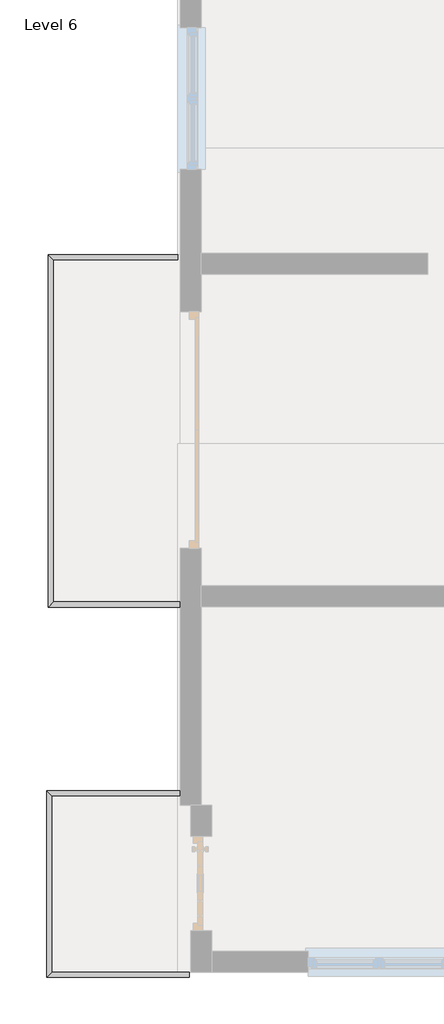
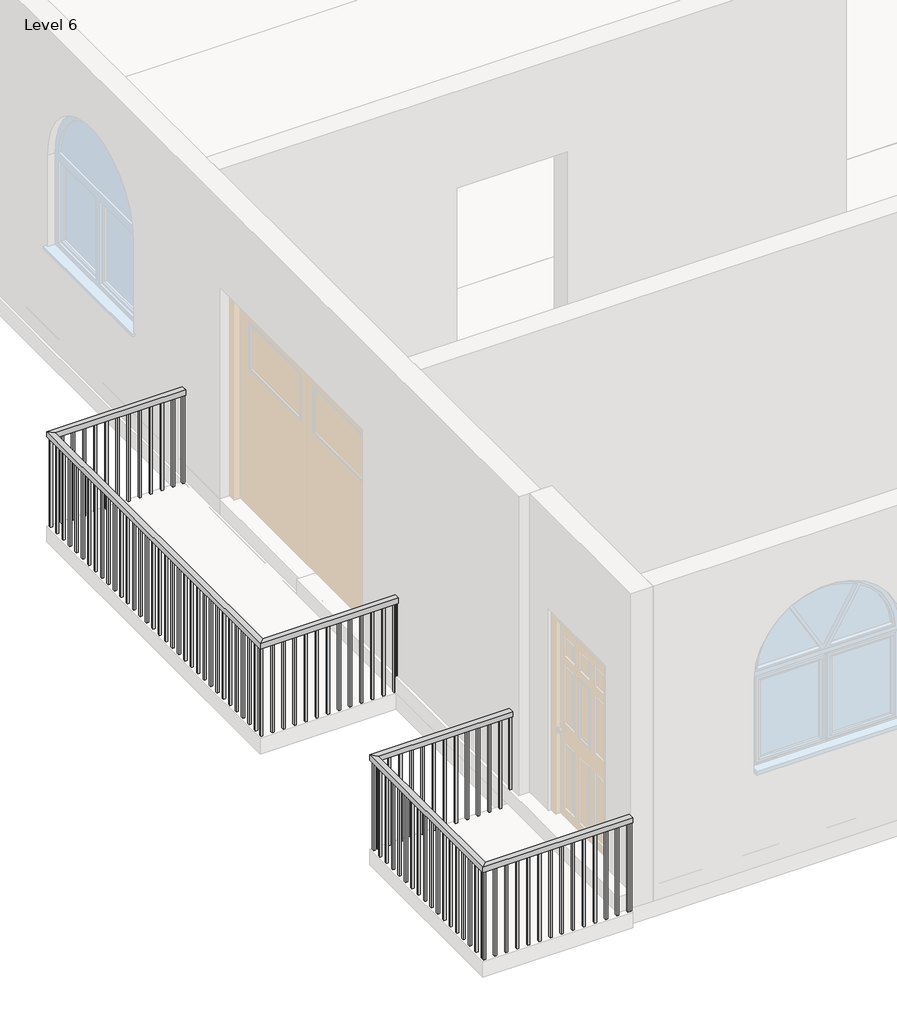
# One storey, part 3 of 7: 2 railings.
"""IFC4 building model written with IfcOpenShell, lengths in millimetres."""

from ifc_helpers import new_model, si_unit, frame, origin, place, context, project, spatial, polyline, outline, extrude, faceted_brep, element, save

model = new_model("IFC4")

# Units and contexts
model_context = context("Model", 3, world=origin())
ifc_project = project(units=[si_unit("LENGTHUNIT", "METRE", prefix="MILLI")], contexts=[model_context])

# Site, building, storey
site = spatial("IfcSite", under=ifc_project)
building = spatial("IfcBuilding", under=site)
storey = spatial("IfcBuildingStorey", under=building, Name="Level 6", Elevation=15240.0)

# Railings
placement = place(None, origin())
element("IfcRailing", 1, ObjectType="Handrail - Rectangular", at=placement, inside=storey, context=model_context, shape_type="SolidModel", body=[
    faceted_brep([(-6354.2109037, -3767.6037749, 16154.4), (-6354.2109037, -3767.6037749, 16103.6), (-6354.2109037, -3716.8037749, 16103.6), (-6354.2109037, -3716.8037749, 16154.4), (-7548.0109037, -3767.6037749, 16154.4), (-7548.0109037, -3767.6037749, 16103.6), (-7598.8109037, -3716.8037749, 16103.6), (-7598.8109037, -3716.8037749, 16154.4), (-7548.0109037, -7054.4894702, 16154.4), (-7548.0109037, -7054.4894702, 16103.6), (-7598.8109037, -7105.2894702, 16103.6), (-7598.8109037, -7105.2894702, 16154.4), (-6330.8013636, -7054.4894702, 16154.4), (-6330.8013636, -7105.2894702, 16154.4), (-6330.8013636, -7105.2894702, 16103.6), (-6330.8013636, -7054.4894702, 16103.6)], [[[0, 1, 2, 3]], [[1, 0, 4, 5]], [[2, 1, 5, 6]], [[3, 2, 6, 7]], [[0, 3, 7, 4]], [[5, 4, 8, 9]], [[6, 5, 9, 10]], [[7, 6, 10, 11]], [[4, 7, 11, 8]], [[12, 13, 14, 15]], [[9, 8, 12, 15]], [[10, 9, 15, 14]], [[11, 10, 14, 13]], [[8, 11, 13, 12]]]),
    extrude(outline(polyline([(-6363.7359037, -7089.4144702), (-6363.7359037, -7070.3644702), (-6344.6859037, -7070.3644702), (-6344.6859037, -7089.4144702), (-6363.7359037, -7089.4144702)])), frame((0.0, 0.0, 15240.0), z_axis=(0.0, 0.0, 1.0), x_axis=(1.0, 0.0, 0.0)), (0.0, 0.0, 1.0), 863.6),
    extrude(outline(polyline([(-6465.3359037, -7089.4144702), (-6465.3359037, -7070.3644702), (-6446.2859037, -7070.3644702), (-6446.2859037, -7089.4144702), (-6465.3359037, -7089.4144702)])), frame((0.0, 0.0, 15240.0), z_axis=(0.0, 0.0, 1.0), x_axis=(1.0, 0.0, 0.0)), (0.0, 0.0, 1.0), 863.6),
    extrude(outline(polyline([(-6566.9359037, -7089.4144702), (-6566.9359037, -7070.3644702), (-6547.8859037, -7070.3644702), (-6547.8859037, -7089.4144702), (-6566.9359037, -7089.4144702)])), frame((0.0, 0.0, 15240.0), z_axis=(0.0, 0.0, 1.0), x_axis=(1.0, 0.0, 0.0)), (0.0, 0.0, 1.0), 863.6),
    extrude(outline(polyline([(-6668.5359037, -7089.4144702), (-6668.5359037, -7070.3644702), (-6649.4859037, -7070.3644702), (-6649.4859037, -7089.4144702), (-6668.5359037, -7089.4144702)])), frame((0.0, 0.0, 15240.0), z_axis=(0.0, 0.0, 1.0), x_axis=(1.0, 0.0, 0.0)), (0.0, 0.0, 1.0), 863.6),
    extrude(outline(polyline([(-6770.1359037, -7089.4144702), (-6770.1359037, -7070.3644702), (-6751.0859037, -7070.3644702), (-6751.0859037, -7089.4144702), (-6770.1359037, -7089.4144702)])), frame((0.0, 0.0, 15240.0), z_axis=(0.0, 0.0, 1.0), x_axis=(1.0, 0.0, 0.0)), (0.0, 0.0, 1.0), 863.6),
    extrude(outline(polyline([(-6871.7359037, -7089.4144702), (-6871.7359037, -7070.3644702), (-6852.6859037, -7070.3644702), (-6852.6859037, -7089.4144702), (-6871.7359037, -7089.4144702)])), frame((0.0, 0.0, 15240.0), z_axis=(0.0, 0.0, 1.0), x_axis=(1.0, 0.0, 0.0)), (0.0, 0.0, 1.0), 863.6),
    extrude(outline(polyline([(-6973.3359037, -7089.4144702), (-6973.3359037, -7070.3644702), (-6954.2859037, -7070.3644702), (-6954.2859037, -7089.4144702), (-6973.3359037, -7089.4144702)])), frame((0.0, 0.0, 15240.0), z_axis=(0.0, 0.0, 1.0), x_axis=(1.0, 0.0, 0.0)), (0.0, 0.0, 1.0), 863.6),
    extrude(outline(polyline([(-7074.9359037, -7089.4144702), (-7074.9359037, -7070.3644702), (-7055.8859037, -7070.3644702), (-7055.8859037, -7089.4144702), (-7074.9359037, -7089.4144702)])), frame((0.0, 0.0, 15240.0), z_axis=(0.0, 0.0, 1.0), x_axis=(1.0, 0.0, 0.0)), (0.0, 0.0, 1.0), 863.6),
    extrude(outline(polyline([(-7176.5359037, -7089.4144702), (-7176.5359037, -7070.3644702), (-7157.4859037, -7070.3644702), (-7157.4859037, -7089.4144702), (-7176.5359037, -7089.4144702)])), frame((0.0, 0.0, 15240.0), z_axis=(0.0, 0.0, 1.0), x_axis=(1.0, 0.0, 0.0)), (0.0, 0.0, 1.0), 863.6),
    extrude(outline(polyline([(-7278.1359037, -7089.4144702), (-7278.1359037, -7070.3644702), (-7259.0859037, -7070.3644702), (-7259.0859037, -7089.4144702), (-7278.1359037, -7089.4144702)])), frame((0.0, 0.0, 15240.0), z_axis=(0.0, 0.0, 1.0), x_axis=(1.0, 0.0, 0.0)), (0.0, 0.0, 1.0), 863.6),
    extrude(outline(polyline([(-7379.7359037, -7089.4144702), (-7379.7359037, -7070.3644702), (-7360.6859037, -7070.3644702), (-7360.6859037, -7089.4144702), (-7379.7359037, -7089.4144702)])), frame((0.0, 0.0, 15240.0), z_axis=(0.0, 0.0, 1.0), x_axis=(1.0, 0.0, 0.0)), (0.0, 0.0, 1.0), 863.6),
    extrude(outline(polyline([(-7481.3359037, -7089.4144702), (-7481.3359037, -7070.3644702), (-7462.2859037, -7070.3644702), (-7462.2859037, -7089.4144702), (-7481.3359037, -7089.4144702)])), frame((0.0, 0.0, 15240.0), z_axis=(0.0, 0.0, 1.0), x_axis=(1.0, 0.0, 0.0)), (0.0, 0.0, 1.0), 863.6),
    extrude(outline(polyline([(-7582.9359037, -6983.8787749), (-7563.8859037, -6983.8787749), (-7563.8859037, -7002.9287749), (-7582.9359037, -7002.9287749), (-7582.9359037, -6983.8787749)])), frame((0.0, 0.0, 15240.0), z_axis=(0.0, 0.0, 1.0), x_axis=(1.0, 0.0, 0.0)), (0.0, 0.0, 1.0), 863.6),
    extrude(outline(polyline([(-7582.9359037, -6882.2787749), (-7563.8859037, -6882.2787749), (-7563.8859037, -6901.3287749), (-7582.9359037, -6901.3287749), (-7582.9359037, -6882.2787749)])), frame((0.0, 0.0, 15240.0), z_axis=(0.0, 0.0, 1.0), x_axis=(1.0, 0.0, 0.0)), (0.0, 0.0, 1.0), 863.6),
    extrude(outline(polyline([(-7582.9359037, -6780.6787749), (-7563.8859037, -6780.6787749), (-7563.8859037, -6799.7287749), (-7582.9359037, -6799.7287749), (-7582.9359037, -6780.6787749)])), frame((0.0, 0.0, 15240.0), z_axis=(0.0, 0.0, 1.0), x_axis=(1.0, 0.0, 0.0)), (0.0, 0.0, 1.0), 863.6),
    extrude(outline(polyline([(-7582.9359037, -6679.0787749), (-7563.8859037, -6679.0787749), (-7563.8859037, -6698.1287749), (-7582.9359037, -6698.1287749), (-7582.9359037, -6679.0787749)])), frame((0.0, 0.0, 15240.0), z_axis=(0.0, 0.0, 1.0), x_axis=(1.0, 0.0, 0.0)), (0.0, 0.0, 1.0), 863.6),
    extrude(outline(polyline([(-7582.9359037, -6577.4787749), (-7563.8859037, -6577.4787749), (-7563.8859037, -6596.5287749), (-7582.9359037, -6596.5287749), (-7582.9359037, -6577.4787749)])), frame((0.0, 0.0, 15240.0), z_axis=(0.0, 0.0, 1.0), x_axis=(1.0, 0.0, 0.0)), (0.0, 0.0, 1.0), 863.6),
    extrude(outline(polyline([(-7582.9359037, -6475.8787749), (-7563.8859037, -6475.8787749), (-7563.8859037, -6494.9287749), (-7582.9359037, -6494.9287749), (-7582.9359037, -6475.8787749)])), frame((0.0, 0.0, 15240.0), z_axis=(0.0, 0.0, 1.0), x_axis=(1.0, 0.0, 0.0)), (0.0, 0.0, 1.0), 863.6),
    extrude(outline(polyline([(-7582.9359037, -6374.2787749), (-7563.8859037, -6374.2787749), (-7563.8859037, -6393.3287749), (-7582.9359037, -6393.3287749), (-7582.9359037, -6374.2787749)])), frame((0.0, 0.0, 15240.0), z_axis=(0.0, 0.0, 1.0), x_axis=(1.0, 0.0, 0.0)), (0.0, 0.0, 1.0), 863.6),
    extrude(outline(polyline([(-7582.9359037, -6272.6787749), (-7563.8859037, -6272.6787749), (-7563.8859037, -6291.7287749), (-7582.9359037, -6291.7287749), (-7582.9359037, -6272.6787749)])), frame((0.0, 0.0, 15240.0), z_axis=(0.0, 0.0, 1.0), x_axis=(1.0, 0.0, 0.0)), (0.0, 0.0, 1.0), 863.6),
    extrude(outline(polyline([(-7582.9359037, -6171.0787749), (-7563.8859037, -6171.0787749), (-7563.8859037, -6190.1287749), (-7582.9359037, -6190.1287749), (-7582.9359037, -6171.0787749)])), frame((0.0, 0.0, 15240.0), z_axis=(0.0, 0.0, 1.0), x_axis=(1.0, 0.0, 0.0)), (0.0, 0.0, 1.0), 863.6),
    extrude(outline(polyline([(-7582.9359037, -6069.4787749), (-7563.8859037, -6069.4787749), (-7563.8859037, -6088.5287749), (-7582.9359037, -6088.5287749), (-7582.9359037, -6069.4787749)])), frame((0.0, 0.0, 15240.0), z_axis=(0.0, 0.0, 1.0), x_axis=(1.0, 0.0, 0.0)), (0.0, 0.0, 1.0), 863.6),
    extrude(outline(polyline([(-7582.9359037, -5967.8787749), (-7563.8859037, -5967.8787749), (-7563.8859037, -5986.9287749), (-7582.9359037, -5986.9287749), (-7582.9359037, -5967.8787749)])), frame((0.0, 0.0, 15240.0), z_axis=(0.0, 0.0, 1.0), x_axis=(1.0, 0.0, 0.0)), (0.0, 0.0, 1.0), 863.6),
    extrude(outline(polyline([(-7582.9359037, -5866.2787749), (-7563.8859037, -5866.2787749), (-7563.8859037, -5885.3287749), (-7582.9359037, -5885.3287749), (-7582.9359037, -5866.2787749)])), frame((0.0, 0.0, 15240.0), z_axis=(0.0, 0.0, 1.0), x_axis=(1.0, 0.0, 0.0)), (0.0, 0.0, 1.0), 863.6),
    extrude(outline(polyline([(-7582.9359037, -5764.6787749), (-7563.8859037, -5764.6787749), (-7563.8859037, -5783.7287749), (-7582.9359037, -5783.7287749), (-7582.9359037, -5764.6787749)])), frame((0.0, 0.0, 15240.0), z_axis=(0.0, 0.0, 1.0), x_axis=(1.0, 0.0, 0.0)), (0.0, 0.0, 1.0), 863.6),
    extrude(outline(polyline([(-7582.9359037, -5663.0787749), (-7563.8859037, -5663.0787749), (-7563.8859037, -5682.1287749), (-7582.9359037, -5682.1287749), (-7582.9359037, -5663.0787749)])), frame((0.0, 0.0, 15240.0), z_axis=(0.0, 0.0, 1.0), x_axis=(1.0, 0.0, 0.0)), (0.0, 0.0, 1.0), 863.6),
    extrude(outline(polyline([(-7582.9359037, -5561.4787749), (-7563.8859037, -5561.4787749), (-7563.8859037, -5580.5287749), (-7582.9359037, -5580.5287749), (-7582.9359037, -5561.4787749)])), frame((0.0, 0.0, 15240.0), z_axis=(0.0, 0.0, 1.0), x_axis=(1.0, 0.0, 0.0)), (0.0, 0.0, 1.0), 863.6),
    extrude(outline(polyline([(-7582.9359037, -5459.8787749), (-7563.8859037, -5459.8787749), (-7563.8859037, -5478.9287749), (-7582.9359037, -5478.9287749), (-7582.9359037, -5459.8787749)])), frame((0.0, 0.0, 15240.0), z_axis=(0.0, 0.0, 1.0), x_axis=(1.0, 0.0, 0.0)), (0.0, 0.0, 1.0), 863.6),
    extrude(outline(polyline([(-7582.9359037, -5358.2787749), (-7563.8859037, -5358.2787749), (-7563.8859037, -5377.3287749), (-7582.9359037, -5377.3287749), (-7582.9359037, -5358.2787749)])), frame((0.0, 0.0, 15240.0), z_axis=(0.0, 0.0, 1.0), x_axis=(1.0, 0.0, 0.0)), (0.0, 0.0, 1.0), 863.6),
    extrude(outline(polyline([(-7582.9359037, -5256.6787749), (-7563.8859037, -5256.6787749), (-7563.8859037, -5275.7287749), (-7582.9359037, -5275.7287749), (-7582.9359037, -5256.6787749)])), frame((0.0, 0.0, 15240.0), z_axis=(0.0, 0.0, 1.0), x_axis=(1.0, 0.0, 0.0)), (0.0, 0.0, 1.0), 863.6),
    extrude(outline(polyline([(-7582.9359037, -5155.0787749), (-7563.8859037, -5155.0787749), (-7563.8859037, -5174.1287749), (-7582.9359037, -5174.1287749), (-7582.9359037, -5155.0787749)])), frame((0.0, 0.0, 15240.0), z_axis=(0.0, 0.0, 1.0), x_axis=(1.0, 0.0, 0.0)), (0.0, 0.0, 1.0), 863.6),
    extrude(outline(polyline([(-7582.9359037, -5053.4787749), (-7563.8859037, -5053.4787749), (-7563.8859037, -5072.5287749), (-7582.9359037, -5072.5287749), (-7582.9359037, -5053.4787749)])), frame((0.0, 0.0, 15240.0), z_axis=(0.0, 0.0, 1.0), x_axis=(1.0, 0.0, 0.0)), (0.0, 0.0, 1.0), 863.6),
    extrude(outline(polyline([(-7582.9359037, -4951.8787749), (-7563.8859037, -4951.8787749), (-7563.8859037, -4970.9287749), (-7582.9359037, -4970.9287749), (-7582.9359037, -4951.8787749)])), frame((0.0, 0.0, 15240.0), z_axis=(0.0, 0.0, 1.0), x_axis=(1.0, 0.0, 0.0)), (0.0, 0.0, 1.0), 863.6),
    extrude(outline(polyline([(-7582.9359037, -4850.2787749), (-7563.8859037, -4850.2787749), (-7563.8859037, -4869.3287749), (-7582.9359037, -4869.3287749), (-7582.9359037, -4850.2787749)])), frame((0.0, 0.0, 15240.0), z_axis=(0.0, 0.0, 1.0), x_axis=(1.0, 0.0, 0.0)), (0.0, 0.0, 1.0), 863.6),
    extrude(outline(polyline([(-7582.9359037, -4748.6787749), (-7563.8859037, -4748.6787749), (-7563.8859037, -4767.7287749), (-7582.9359037, -4767.7287749), (-7582.9359037, -4748.6787749)])), frame((0.0, 0.0, 15240.0), z_axis=(0.0, 0.0, 1.0), x_axis=(1.0, 0.0, 0.0)), (0.0, 0.0, 1.0), 863.6),
    extrude(outline(polyline([(-7582.9359037, -4647.0787749), (-7563.8859037, -4647.0787749), (-7563.8859037, -4666.1287749), (-7582.9359037, -4666.1287749), (-7582.9359037, -4647.0787749)])), frame((0.0, 0.0, 15240.0), z_axis=(0.0, 0.0, 1.0), x_axis=(1.0, 0.0, 0.0)), (0.0, 0.0, 1.0), 863.6),
    extrude(outline(polyline([(-7582.9359037, -4545.4787749), (-7563.8859037, -4545.4787749), (-7563.8859037, -4564.5287749), (-7582.9359037, -4564.5287749), (-7582.9359037, -4545.4787749)])), frame((0.0, 0.0, 15240.0), z_axis=(0.0, 0.0, 1.0), x_axis=(1.0, 0.0, 0.0)), (0.0, 0.0, 1.0), 863.6),
    extrude(outline(polyline([(-7582.9359037, -4443.8787749), (-7563.8859037, -4443.8787749), (-7563.8859037, -4462.9287749), (-7582.9359037, -4462.9287749), (-7582.9359037, -4443.8787749)])), frame((0.0, 0.0, 15240.0), z_axis=(0.0, 0.0, 1.0), x_axis=(1.0, 0.0, 0.0)), (0.0, 0.0, 1.0), 863.6),
    extrude(outline(polyline([(-7582.9359037, -4342.2787749), (-7563.8859037, -4342.2787749), (-7563.8859037, -4361.3287749), (-7582.9359037, -4361.3287749), (-7582.9359037, -4342.2787749)])), frame((0.0, 0.0, 15240.0), z_axis=(0.0, 0.0, 1.0), x_axis=(1.0, 0.0, 0.0)), (0.0, 0.0, 1.0), 863.6),
    extrude(outline(polyline([(-7582.9359037, -4240.6787749), (-7563.8859037, -4240.6787749), (-7563.8859037, -4259.7287749), (-7582.9359037, -4259.7287749), (-7582.9359037, -4240.6787749)])), frame((0.0, 0.0, 15240.0), z_axis=(0.0, 0.0, 1.0), x_axis=(1.0, 0.0, 0.0)), (0.0, 0.0, 1.0), 863.6),
    extrude(outline(polyline([(-7582.9359037, -4139.0787749), (-7563.8859037, -4139.0787749), (-7563.8859037, -4158.1287749), (-7582.9359037, -4158.1287749), (-7582.9359037, -4139.0787749)])), frame((0.0, 0.0, 15240.0), z_axis=(0.0, 0.0, 1.0), x_axis=(1.0, 0.0, 0.0)), (0.0, 0.0, 1.0), 863.6),
    extrude(outline(polyline([(-7582.9359037, -4037.4787749), (-7563.8859037, -4037.4787749), (-7563.8859037, -4056.5287749), (-7582.9359037, -4056.5287749), (-7582.9359037, -4037.4787749)])), frame((0.0, 0.0, 15240.0), z_axis=(0.0, 0.0, 1.0), x_axis=(1.0, 0.0, 0.0)), (0.0, 0.0, 1.0), 863.6),
    extrude(outline(polyline([(-7582.9359037, -3935.8787749), (-7563.8859037, -3935.8787749), (-7563.8859037, -3954.9287749), (-7582.9359037, -3954.9287749), (-7582.9359037, -3935.8787749)])), frame((0.0, 0.0, 15240.0), z_axis=(0.0, 0.0, 1.0), x_axis=(1.0, 0.0, 0.0)), (0.0, 0.0, 1.0), 863.6),
    extrude(outline(polyline([(-7582.9359037, -3834.2787749), (-7563.8859037, -3834.2787749), (-7563.8859037, -3853.3287749), (-7582.9359037, -3853.3287749), (-7582.9359037, -3834.2787749)])), frame((0.0, 0.0, 15240.0), z_axis=(0.0, 0.0, 1.0), x_axis=(1.0, 0.0, 0.0)), (0.0, 0.0, 1.0), 863.6),
    extrude(outline(polyline([(-7462.2859037, -3732.6787749), (-7462.2859037, -3751.7287749), (-7481.3359037, -3751.7287749), (-7481.3359037, -3732.6787749), (-7462.2859037, -3732.6787749)])), frame((0.0, 0.0, 15240.0), z_axis=(0.0, 0.0, 1.0), x_axis=(1.0, 0.0, 0.0)), (0.0, 0.0, 1.0), 863.6),
    extrude(outline(polyline([(-7360.6859037, -3732.6787749), (-7360.6859037, -3751.7287749), (-7379.7359037, -3751.7287749), (-7379.7359037, -3732.6787749), (-7360.6859037, -3732.6787749)])), frame((0.0, 0.0, 15240.0), z_axis=(0.0, 0.0, 1.0), x_axis=(1.0, 0.0, 0.0)), (0.0, 0.0, 1.0), 863.6),
    extrude(outline(polyline([(-7259.0859037, -3732.6787749), (-7259.0859037, -3751.7287749), (-7278.1359037, -3751.7287749), (-7278.1359037, -3732.6787749), (-7259.0859037, -3732.6787749)])), frame((0.0, 0.0, 15240.0), z_axis=(0.0, 0.0, 1.0), x_axis=(1.0, 0.0, 0.0)), (0.0, 0.0, 1.0), 863.6),
    extrude(outline(polyline([(-7157.4859037, -3732.6787749), (-7157.4859037, -3751.7287749), (-7176.5359037, -3751.7287749), (-7176.5359037, -3732.6787749), (-7157.4859037, -3732.6787749)])), frame((0.0, 0.0, 15240.0), z_axis=(0.0, 0.0, 1.0), x_axis=(1.0, 0.0, 0.0)), (0.0, 0.0, 1.0), 863.6),
    extrude(outline(polyline([(-7055.8859037, -3732.6787749), (-7055.8859037, -3751.7287749), (-7074.9359037, -3751.7287749), (-7074.9359037, -3732.6787749), (-7055.8859037, -3732.6787749)])), frame((0.0, 0.0, 15240.0), z_axis=(0.0, 0.0, 1.0), x_axis=(1.0, 0.0, 0.0)), (0.0, 0.0, 1.0), 863.6),
    extrude(outline(polyline([(-6954.2859037, -3732.6787749), (-6954.2859037, -3751.7287749), (-6973.3359037, -3751.7287749), (-6973.3359037, -3732.6787749), (-6954.2859037, -3732.6787749)])), frame((0.0, 0.0, 15240.0), z_axis=(0.0, 0.0, 1.0), x_axis=(1.0, 0.0, 0.0)), (0.0, 0.0, 1.0), 863.6),
    extrude(outline(polyline([(-6852.6859037, -3732.6787749), (-6852.6859037, -3751.7287749), (-6871.7359037, -3751.7287749), (-6871.7359037, -3732.6787749), (-6852.6859037, -3732.6787749)])), frame((0.0, 0.0, 15240.0), z_axis=(0.0, 0.0, 1.0), x_axis=(1.0, 0.0, 0.0)), (0.0, 0.0, 1.0), 863.6),
    extrude(outline(polyline([(-6751.0859037, -3732.6787749), (-6751.0859037, -3751.7287749), (-6770.1359037, -3751.7287749), (-6770.1359037, -3732.6787749), (-6751.0859037, -3732.6787749)])), frame((0.0, 0.0, 15240.0), z_axis=(0.0, 0.0, 1.0), x_axis=(1.0, 0.0, 0.0)), (0.0, 0.0, 1.0), 863.6),
    extrude(outline(polyline([(-6649.4859037, -3732.6787749), (-6649.4859037, -3751.7287749), (-6668.5359037, -3751.7287749), (-6668.5359037, -3732.6787749), (-6649.4859037, -3732.6787749)])), frame((0.0, 0.0, 15240.0), z_axis=(0.0, 0.0, 1.0), x_axis=(1.0, 0.0, 0.0)), (0.0, 0.0, 1.0), 863.6),
    extrude(outline(polyline([(-6547.8859037, -3732.6787749), (-6547.8859037, -3751.7287749), (-6566.9359037, -3751.7287749), (-6566.9359037, -3732.6787749), (-6547.8859037, -3732.6787749)])), frame((0.0, 0.0, 15240.0), z_axis=(0.0, 0.0, 1.0), x_axis=(1.0, 0.0, 0.0)), (0.0, 0.0, 1.0), 863.6),
    extrude(outline(polyline([(-6446.2859037, -3732.6787749), (-6446.2859037, -3751.7287749), (-6465.3359037, -3751.7287749), (-6465.3359037, -3732.6787749), (-6446.2859037, -3732.6787749)])), frame((0.0, 0.0, 15240.0), z_axis=(0.0, 0.0, 1.0), x_axis=(1.0, 0.0, 0.0)), (0.0, 0.0, 1.0), 863.6),
    extrude(outline(polyline([(-7582.9359037, -7070.3644702), (-7563.8859037, -7070.3644702), (-7563.8859037, -7089.4144702), (-7582.9359037, -7089.4144702), (-7582.9359037, -7070.3644702)])), frame((0.0, 0.0, 15240.0), z_axis=(0.0, 0.0, 1.0), x_axis=(1.0, 0.0, 0.0)), (0.0, 0.0, 1.0), 863.6),
    extrude(outline(polyline([(-7563.8859037, -3732.6787749), (-7563.8859037, -3751.7287749), (-7582.9359037, -3751.7287749), (-7582.9359037, -3732.6787749), (-7563.8859037, -3732.6787749)])), frame((0.0, 0.0, 15240.0), z_axis=(0.0, 0.0, 1.0), x_axis=(1.0, 0.0, 0.0)), (0.0, 0.0, 1.0), 863.6),
    extrude(outline(polyline([(-6349.8513636, -7089.4144702), (-6349.8513636, -7070.3644702), (-6330.8013636, -7070.3644702), (-6330.8013636, -7089.4144702), (-6349.8513636, -7089.4144702)])), frame((0.0, 0.0, 15240.0), z_axis=(0.0, 0.0, 1.0), x_axis=(1.0, 0.0, 0.0)), (0.0, 0.0, 1.0), 863.6),
    extrude(outline(polyline([(-6354.2109037, -3732.6787749), (-6354.2109037, -3751.7287749), (-6373.2609037, -3751.7287749), (-6373.2609037, -3732.6787749), (-6354.2109037, -3732.6787749)])), frame((0.0, 0.0, 15240.0), z_axis=(0.0, 0.0, 1.0), x_axis=(1.0, 0.0, 0.0)), (0.0, 0.0, 1.0), 863.6),
])
element("IfcRailing", 2, ObjectType="Handrail - Rectangular", at=placement, inside=storey, context=model_context, shape_type="SolidModel", body=[
    faceted_brep([(-6330.8013636, -8918.8845215, 16154.4), (-6330.8013636, -8918.8845215, 16103.6), (-6330.8013636, -8868.0845215, 16103.6), (-6330.8013636, -8868.0845215, 16154.4), (-7563.8859037, -8918.8845215, 16154.4), (-7563.8859037, -8918.8845215, 16103.6), (-7614.6859037, -8868.0845215, 16103.6), (-7614.6859037, -8868.0845215, 16154.4), (-7563.8859037, -10612.9037749, 16154.4), (-7563.8859037, -10612.9037749, 16103.6), (-7614.6859037, -10663.7037749, 16103.6), (-7614.6859037, -10663.7037749, 16154.4), (-6243.0859037, -10612.9037749, 16154.4), (-6243.0859037, -10663.7037749, 16154.4), (-6243.0859037, -10663.7037749, 16103.6), (-6243.0859037, -10612.9037749, 16103.6)], [[[0, 1, 2, 3]], [[1, 0, 4, 5]], [[2, 1, 5, 6]], [[3, 2, 6, 7]], [[0, 3, 7, 4]], [[5, 4, 8, 9]], [[6, 5, 9, 10]], [[7, 6, 10, 11]], [[4, 7, 11, 8]], [[12, 13, 14, 15]], [[9, 8, 12, 15]], [[10, 9, 15, 14]], [[11, 10, 14, 13]], [[8, 11, 13, 12]]]),
    extrude(outline(polyline([(-6278.0109037, -10647.8287749), (-6278.0109037, -10628.7787749), (-6258.9609037, -10628.7787749), (-6258.9609037, -10647.8287749), (-6278.0109037, -10647.8287749)])), frame((0.0, 0.0, 15240.0), z_axis=(0.0, 0.0, 1.0), x_axis=(1.0, 0.0, 0.0)), (0.0, 0.0, 1.0), 863.6),
    extrude(outline(polyline([(-6379.6109037, -10647.8287749), (-6379.6109037, -10628.7787749), (-6360.5609037, -10628.7787749), (-6360.5609037, -10647.8287749), (-6379.6109037, -10647.8287749)])), frame((0.0, 0.0, 15240.0), z_axis=(0.0, 0.0, 1.0), x_axis=(1.0, 0.0, 0.0)), (0.0, 0.0, 1.0), 863.6),
    extrude(outline(polyline([(-6481.2109037, -10647.8287749), (-6481.2109037, -10628.7787749), (-6462.1609037, -10628.7787749), (-6462.1609037, -10647.8287749), (-6481.2109037, -10647.8287749)])), frame((0.0, 0.0, 15240.0), z_axis=(0.0, 0.0, 1.0), x_axis=(1.0, 0.0, 0.0)), (0.0, 0.0, 1.0), 863.6),
    extrude(outline(polyline([(-6582.8109037, -10647.8287749), (-6582.8109037, -10628.7787749), (-6563.7609037, -10628.7787749), (-6563.7609037, -10647.8287749), (-6582.8109037, -10647.8287749)])), frame((0.0, 0.0, 15240.0), z_axis=(0.0, 0.0, 1.0), x_axis=(1.0, 0.0, 0.0)), (0.0, 0.0, 1.0), 863.6),
    extrude(outline(polyline([(-6684.4109037, -10647.8287749), (-6684.4109037, -10628.7787749), (-6665.3609037, -10628.7787749), (-6665.3609037, -10647.8287749), (-6684.4109037, -10647.8287749)])), frame((0.0, 0.0, 15240.0), z_axis=(0.0, 0.0, 1.0), x_axis=(1.0, 0.0, 0.0)), (0.0, 0.0, 1.0), 863.6),
    extrude(outline(polyline([(-6786.0109037, -10647.8287749), (-6786.0109037, -10628.7787749), (-6766.9609037, -10628.7787749), (-6766.9609037, -10647.8287749), (-6786.0109037, -10647.8287749)])), frame((0.0, 0.0, 15240.0), z_axis=(0.0, 0.0, 1.0), x_axis=(1.0, 0.0, 0.0)), (0.0, 0.0, 1.0), 863.6),
    extrude(outline(polyline([(-6887.6109037, -10647.8287749), (-6887.6109037, -10628.7787749), (-6868.5609037, -10628.7787749), (-6868.5609037, -10647.8287749), (-6887.6109037, -10647.8287749)])), frame((0.0, 0.0, 15240.0), z_axis=(0.0, 0.0, 1.0), x_axis=(1.0, 0.0, 0.0)), (0.0, 0.0, 1.0), 863.6),
    extrude(outline(polyline([(-6989.2109037, -10647.8287749), (-6989.2109037, -10628.7787749), (-6970.1609037, -10628.7787749), (-6970.1609037, -10647.8287749), (-6989.2109037, -10647.8287749)])), frame((0.0, 0.0, 15240.0), z_axis=(0.0, 0.0, 1.0), x_axis=(1.0, 0.0, 0.0)), (0.0, 0.0, 1.0), 863.6),
    extrude(outline(polyline([(-7090.8109037, -10647.8287749), (-7090.8109037, -10628.7787749), (-7071.7609037, -10628.7787749), (-7071.7609037, -10647.8287749), (-7090.8109037, -10647.8287749)])), frame((0.0, 0.0, 15240.0), z_axis=(0.0, 0.0, 1.0), x_axis=(1.0, 0.0, 0.0)), (0.0, 0.0, 1.0), 863.6),
    extrude(outline(polyline([(-7192.4109037, -10647.8287749), (-7192.4109037, -10628.7787749), (-7173.3609037, -10628.7787749), (-7173.3609037, -10647.8287749), (-7192.4109037, -10647.8287749)])), frame((0.0, 0.0, 15240.0), z_axis=(0.0, 0.0, 1.0), x_axis=(1.0, 0.0, 0.0)), (0.0, 0.0, 1.0), 863.6),
    extrude(outline(polyline([(-7294.0109037, -10647.8287749), (-7294.0109037, -10628.7787749), (-7274.9609037, -10628.7787749), (-7274.9609037, -10647.8287749), (-7294.0109037, -10647.8287749)])), frame((0.0, 0.0, 15240.0), z_axis=(0.0, 0.0, 1.0), x_axis=(1.0, 0.0, 0.0)), (0.0, 0.0, 1.0), 863.6),
    extrude(outline(polyline([(-7395.6109037, -10647.8287749), (-7395.6109037, -10628.7787749), (-7376.5609037, -10628.7787749), (-7376.5609037, -10647.8287749), (-7395.6109037, -10647.8287749)])), frame((0.0, 0.0, 15240.0), z_axis=(0.0, 0.0, 1.0), x_axis=(1.0, 0.0, 0.0)), (0.0, 0.0, 1.0), 863.6),
    extrude(outline(polyline([(-7497.2109037, -10647.8287749), (-7497.2109037, -10628.7787749), (-7478.1609037, -10628.7787749), (-7478.1609037, -10647.8287749), (-7497.2109037, -10647.8287749)])), frame((0.0, 0.0, 15240.0), z_axis=(0.0, 0.0, 1.0), x_axis=(1.0, 0.0, 0.0)), (0.0, 0.0, 1.0), 863.6),
    extrude(outline(polyline([(-7598.8109037, -10611.1595215), (-7579.7609037, -10611.1595215), (-7579.7609037, -10630.2095215), (-7598.8109037, -10630.2095215), (-7598.8109037, -10611.1595215)])), frame((0.0, 0.0, 15240.0), z_axis=(0.0, 0.0, 1.0), x_axis=(1.0, 0.0, 0.0)), (0.0, 0.0, 1.0), 863.6),
    extrude(outline(polyline([(-7598.8109037, -10509.5595215), (-7579.7609037, -10509.5595215), (-7579.7609037, -10528.6095215), (-7598.8109037, -10528.6095215), (-7598.8109037, -10509.5595215)])), frame((0.0, 0.0, 15240.0), z_axis=(0.0, 0.0, 1.0), x_axis=(1.0, 0.0, 0.0)), (0.0, 0.0, 1.0), 863.6),
    extrude(outline(polyline([(-7598.8109037, -10407.9595215), (-7579.7609037, -10407.9595215), (-7579.7609037, -10427.0095215), (-7598.8109037, -10427.0095215), (-7598.8109037, -10407.9595215)])), frame((0.0, 0.0, 15240.0), z_axis=(0.0, 0.0, 1.0), x_axis=(1.0, 0.0, 0.0)), (0.0, 0.0, 1.0), 863.6),
    extrude(outline(polyline([(-7598.8109037, -10306.3595215), (-7579.7609037, -10306.3595215), (-7579.7609037, -10325.4095215), (-7598.8109037, -10325.4095215), (-7598.8109037, -10306.3595215)])), frame((0.0, 0.0, 15240.0), z_axis=(0.0, 0.0, 1.0), x_axis=(1.0, 0.0, 0.0)), (0.0, 0.0, 1.0), 863.6),
    extrude(outline(polyline([(-7598.8109037, -10204.7595215), (-7579.7609037, -10204.7595215), (-7579.7609037, -10223.8095215), (-7598.8109037, -10223.8095215), (-7598.8109037, -10204.7595215)])), frame((0.0, 0.0, 15240.0), z_axis=(0.0, 0.0, 1.0), x_axis=(1.0, 0.0, 0.0)), (0.0, 0.0, 1.0), 863.6),
    extrude(outline(polyline([(-7598.8109037, -10103.1595215), (-7579.7609037, -10103.1595215), (-7579.7609037, -10122.2095215), (-7598.8109037, -10122.2095215), (-7598.8109037, -10103.1595215)])), frame((0.0, 0.0, 15240.0), z_axis=(0.0, 0.0, 1.0), x_axis=(1.0, 0.0, 0.0)), (0.0, 0.0, 1.0), 863.6),
    extrude(outline(polyline([(-7598.8109037, -10001.5595215), (-7579.7609037, -10001.5595215), (-7579.7609037, -10020.6095215), (-7598.8109037, -10020.6095215), (-7598.8109037, -10001.5595215)])), frame((0.0, 0.0, 15240.0), z_axis=(0.0, 0.0, 1.0), x_axis=(1.0, 0.0, 0.0)), (0.0, 0.0, 1.0), 863.6),
    extrude(outline(polyline([(-7598.8109037, -9899.9595215), (-7579.7609037, -9899.9595215), (-7579.7609037, -9919.0095215), (-7598.8109037, -9919.0095215), (-7598.8109037, -9899.9595215)])), frame((0.0, 0.0, 15240.0), z_axis=(0.0, 0.0, 1.0), x_axis=(1.0, 0.0, 0.0)), (0.0, 0.0, 1.0), 863.6),
    extrude(outline(polyline([(-7598.8109037, -9798.3595215), (-7579.7609037, -9798.3595215), (-7579.7609037, -9817.4095215), (-7598.8109037, -9817.4095215), (-7598.8109037, -9798.3595215)])), frame((0.0, 0.0, 15240.0), z_axis=(0.0, 0.0, 1.0), x_axis=(1.0, 0.0, 0.0)), (0.0, 0.0, 1.0), 863.6),
    extrude(outline(polyline([(-7598.8109037, -9696.7595215), (-7579.7609037, -9696.7595215), (-7579.7609037, -9715.8095215), (-7598.8109037, -9715.8095215), (-7598.8109037, -9696.7595215)])), frame((0.0, 0.0, 15240.0), z_axis=(0.0, 0.0, 1.0), x_axis=(1.0, 0.0, 0.0)), (0.0, 0.0, 1.0), 863.6),
    extrude(outline(polyline([(-7598.8109037, -9595.1595215), (-7579.7609037, -9595.1595215), (-7579.7609037, -9614.2095215), (-7598.8109037, -9614.2095215), (-7598.8109037, -9595.1595215)])), frame((0.0, 0.0, 15240.0), z_axis=(0.0, 0.0, 1.0), x_axis=(1.0, 0.0, 0.0)), (0.0, 0.0, 1.0), 863.6),
    extrude(outline(polyline([(-7598.8109037, -9493.5595215), (-7579.7609037, -9493.5595215), (-7579.7609037, -9512.6095215), (-7598.8109037, -9512.6095215), (-7598.8109037, -9493.5595215)])), frame((0.0, 0.0, 15240.0), z_axis=(0.0, 0.0, 1.0), x_axis=(1.0, 0.0, 0.0)), (0.0, 0.0, 1.0), 863.6),
    extrude(outline(polyline([(-7598.8109037, -9391.9595215), (-7579.7609037, -9391.9595215), (-7579.7609037, -9411.0095215), (-7598.8109037, -9411.0095215), (-7598.8109037, -9391.9595215)])), frame((0.0, 0.0, 15240.0), z_axis=(0.0, 0.0, 1.0), x_axis=(1.0, 0.0, 0.0)), (0.0, 0.0, 1.0), 863.6),
    extrude(outline(polyline([(-7598.8109037, -9290.3595215), (-7579.7609037, -9290.3595215), (-7579.7609037, -9309.4095215), (-7598.8109037, -9309.4095215), (-7598.8109037, -9290.3595215)])), frame((0.0, 0.0, 15240.0), z_axis=(0.0, 0.0, 1.0), x_axis=(1.0, 0.0, 0.0)), (0.0, 0.0, 1.0), 863.6),
    extrude(outline(polyline([(-7598.8109037, -9188.7595215), (-7579.7609037, -9188.7595215), (-7579.7609037, -9207.8095215), (-7598.8109037, -9207.8095215), (-7598.8109037, -9188.7595215)])), frame((0.0, 0.0, 15240.0), z_axis=(0.0, 0.0, 1.0), x_axis=(1.0, 0.0, 0.0)), (0.0, 0.0, 1.0), 863.6),
    extrude(outline(polyline([(-7598.8109037, -9087.1595215), (-7579.7609037, -9087.1595215), (-7579.7609037, -9106.2095215), (-7598.8109037, -9106.2095215), (-7598.8109037, -9087.1595215)])), frame((0.0, 0.0, 15240.0), z_axis=(0.0, 0.0, 1.0), x_axis=(1.0, 0.0, 0.0)), (0.0, 0.0, 1.0), 863.6),
    extrude(outline(polyline([(-7598.8109037, -8985.5595215), (-7579.7609037, -8985.5595215), (-7579.7609037, -9004.6095215), (-7598.8109037, -9004.6095215), (-7598.8109037, -8985.5595215)])), frame((0.0, 0.0, 15240.0), z_axis=(0.0, 0.0, 1.0), x_axis=(1.0, 0.0, 0.0)), (0.0, 0.0, 1.0), 863.6),
    extrude(outline(polyline([(-7540.4763636, -8883.9595215), (-7540.4763636, -8903.0095215), (-7559.5263636, -8903.0095215), (-7559.5263636, -8883.9595215), (-7540.4763636, -8883.9595215)])), frame((0.0, 0.0, 15240.0), z_axis=(0.0, 0.0, 1.0), x_axis=(1.0, 0.0, 0.0)), (0.0, 0.0, 1.0), 863.6),
    extrude(outline(polyline([(-7438.8763636, -8883.9595215), (-7438.8763636, -8903.0095215), (-7457.9263636, -8903.0095215), (-7457.9263636, -8883.9595215), (-7438.8763636, -8883.9595215)])), frame((0.0, 0.0, 15240.0), z_axis=(0.0, 0.0, 1.0), x_axis=(1.0, 0.0, 0.0)), (0.0, 0.0, 1.0), 863.6),
    extrude(outline(polyline([(-7337.2763636, -8883.9595215), (-7337.2763636, -8903.0095215), (-7356.3263636, -8903.0095215), (-7356.3263636, -8883.9595215), (-7337.2763636, -8883.9595215)])), frame((0.0, 0.0, 15240.0), z_axis=(0.0, 0.0, 1.0), x_axis=(1.0, 0.0, 0.0)), (0.0, 0.0, 1.0), 863.6),
    extrude(outline(polyline([(-7235.6763636, -8883.9595215), (-7235.6763636, -8903.0095215), (-7254.7263636, -8903.0095215), (-7254.7263636, -8883.9595215), (-7235.6763636, -8883.9595215)])), frame((0.0, 0.0, 15240.0), z_axis=(0.0, 0.0, 1.0), x_axis=(1.0, 0.0, 0.0)), (0.0, 0.0, 1.0), 863.6),
    extrude(outline(polyline([(-7134.0763636, -8883.9595215), (-7134.0763636, -8903.0095215), (-7153.1263636, -8903.0095215), (-7153.1263636, -8883.9595215), (-7134.0763636, -8883.9595215)])), frame((0.0, 0.0, 15240.0), z_axis=(0.0, 0.0, 1.0), x_axis=(1.0, 0.0, 0.0)), (0.0, 0.0, 1.0), 863.6),
    extrude(outline(polyline([(-7032.4763636, -8883.9595215), (-7032.4763636, -8903.0095215), (-7051.5263636, -8903.0095215), (-7051.5263636, -8883.9595215), (-7032.4763636, -8883.9595215)])), frame((0.0, 0.0, 15240.0), z_axis=(0.0, 0.0, 1.0), x_axis=(1.0, 0.0, 0.0)), (0.0, 0.0, 1.0), 863.6),
    extrude(outline(polyline([(-6930.8763636, -8883.9595215), (-6930.8763636, -8903.0095215), (-6949.9263636, -8903.0095215), (-6949.9263636, -8883.9595215), (-6930.8763636, -8883.9595215)])), frame((0.0, 0.0, 15240.0), z_axis=(0.0, 0.0, 1.0), x_axis=(1.0, 0.0, 0.0)), (0.0, 0.0, 1.0), 863.6),
    extrude(outline(polyline([(-6829.2763636, -8883.9595215), (-6829.2763636, -8903.0095215), (-6848.3263636, -8903.0095215), (-6848.3263636, -8883.9595215), (-6829.2763636, -8883.9595215)])), frame((0.0, 0.0, 15240.0), z_axis=(0.0, 0.0, 1.0), x_axis=(1.0, 0.0, 0.0)), (0.0, 0.0, 1.0), 863.6),
    extrude(outline(polyline([(-6727.6763636, -8883.9595215), (-6727.6763636, -8903.0095215), (-6746.7263636, -8903.0095215), (-6746.7263636, -8883.9595215), (-6727.6763636, -8883.9595215)])), frame((0.0, 0.0, 15240.0), z_axis=(0.0, 0.0, 1.0), x_axis=(1.0, 0.0, 0.0)), (0.0, 0.0, 1.0), 863.6),
    extrude(outline(polyline([(-6626.0763636, -8883.9595215), (-6626.0763636, -8903.0095215), (-6645.1263636, -8903.0095215), (-6645.1263636, -8883.9595215), (-6626.0763636, -8883.9595215)])), frame((0.0, 0.0, 15240.0), z_axis=(0.0, 0.0, 1.0), x_axis=(1.0, 0.0, 0.0)), (0.0, 0.0, 1.0), 863.6),
    extrude(outline(polyline([(-6524.4763636, -8883.9595215), (-6524.4763636, -8903.0095215), (-6543.5263636, -8903.0095215), (-6543.5263636, -8883.9595215), (-6524.4763636, -8883.9595215)])), frame((0.0, 0.0, 15240.0), z_axis=(0.0, 0.0, 1.0), x_axis=(1.0, 0.0, 0.0)), (0.0, 0.0, 1.0), 863.6),
    extrude(outline(polyline([(-6422.8763636, -8883.9595215), (-6422.8763636, -8903.0095215), (-6441.9263636, -8903.0095215), (-6441.9263636, -8883.9595215), (-6422.8763636, -8883.9595215)])), frame((0.0, 0.0, 15240.0), z_axis=(0.0, 0.0, 1.0), x_axis=(1.0, 0.0, 0.0)), (0.0, 0.0, 1.0), 863.6),
    extrude(outline(polyline([(-7598.8109037, -10628.7787749), (-7579.7609037, -10628.7787749), (-7579.7609037, -10647.8287749), (-7598.8109037, -10647.8287749), (-7598.8109037, -10628.7787749)])), frame((0.0, 0.0, 15240.0), z_axis=(0.0, 0.0, 1.0), x_axis=(1.0, 0.0, 0.0)), (0.0, 0.0, 1.0), 863.6),
    extrude(outline(polyline([(-7579.7609037, -8883.9595215), (-7579.7609037, -8903.0095215), (-7598.8109037, -8903.0095215), (-7598.8109037, -8883.9595215), (-7579.7609037, -8883.9595215)])), frame((0.0, 0.0, 15240.0), z_axis=(0.0, 0.0, 1.0), x_axis=(1.0, 0.0, 0.0)), (0.0, 0.0, 1.0), 863.6),
    extrude(outline(polyline([(-6262.1359037, -10647.8287749), (-6262.1359037, -10628.7787749), (-6243.0859037, -10628.7787749), (-6243.0859037, -10647.8287749), (-6262.1359037, -10647.8287749)])), frame((0.0, 0.0, 15240.0), z_axis=(0.0, 0.0, 1.0), x_axis=(1.0, 0.0, 0.0)), (0.0, 0.0, 1.0), 863.6),
    extrude(outline(polyline([(-6330.8013636, -8883.9595215), (-6330.8013636, -8903.0095215), (-6349.8513636, -8903.0095215), (-6349.8513636, -8883.9595215), (-6330.8013636, -8883.9595215)])), frame((0.0, 0.0, 15240.0), z_axis=(0.0, 0.0, 1.0), x_axis=(1.0, 0.0, 0.0)), (0.0, 0.0, 1.0), 863.6),
])

save(model, "model.ifc")

# Revit data of these elements
# Type "Handrail - Rectangular"
#   Assembly Code = "C2010400"
#   built-in parameter 1008612 = 0.0416667 (stored number, unit not read)
#   built-in parameter 1008611 = 0.0416667 (stored number, unit not read)
#   built-in parameter 1008609 = 0.333333 (stored number, unit not read)
#   built-in parameter 1008604 = 0.166667 (stored number, unit not read)
#   built-in parameter 1008603 = 0.166667 (stored number, unit not read)
#   Railing Height = 3' - 0"
#   built-in parameter 1008630 = 2
#   built-in parameter 1008610 = 2
#   built-in parameter 1008618 = Baluster - Square : 3/4"
# Elements 1, 2 (IfcRailing, "Handrail - Rectangular")
#   Phase Created = New Construction
